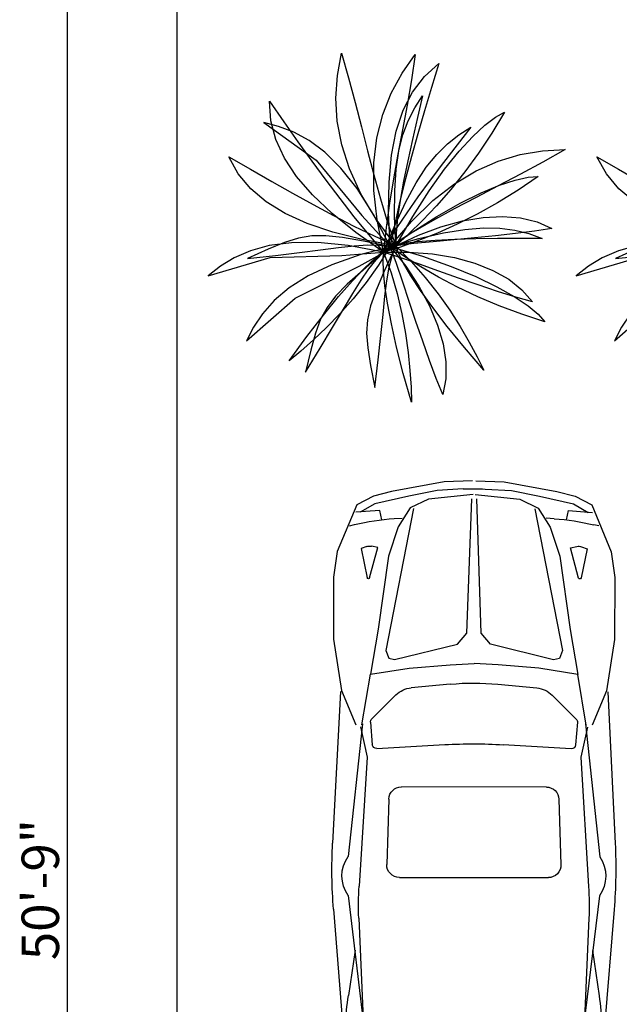
# Model space of a CAD drawing. Units: inches. Extents: x 3394 to 4794, y 965 to 1718.
# Tile 6 of 15: x 3394 to 3522, y 1338 to 1548. Entities that reach past the tile are written whole.
import ezdxf

# ---------------------------------------------------------------- set-up
doc = ezdxf.new("R2010")
doc.units = ezdxf.units.IN
for name, color, linetype, lineweight in [('A-ANNO-DIMS', 2, 'Continuous', 13), ('C-PRKG-VEHI', 8, 'Continuous', 13), ('C-PROP', 7, 'Continuous', 25), ('CAY', 94, 'Continuous', 13)]:
    doc.layers.add(name, color=color, linetype=linetype, lineweight=lineweight)
doc.layers.add('DIENHOA', color=3, linetype='Continuous')
doc.layers.add('L9012X$0', color=2, linetype='Continuous')
doc.styles.get("Standard").update_dxf_attribs({"font": 'arial.ttf'})
doc.dimstyles.new('ISO-25', dxfattribs={"dimtxt": 8, "dimasz": 2.5, "dimexe": 1.25, "dimexo": 0.625, "dimtad": 1, "dimlunit": 3, "dimtxsty": 'Standard', "dimcen": 2.5, "dimadec": 0, "dimazin": 0, "dimtfac": 1, "dimtmove": 0, "dimatfit": 3, "dimfxl": 1, "dimarcsym": 0})

# ---------------------------------------------------------------- blocks, each defined once
blk = doc.blocks.new('A1099DC')
at = {"color": 0, "linetype": 'ByBlock'}
for p, q in [((1279.298465, 804.448389), (2201.430588, 851.890505)), ((2602.736326, 846.078152), (3356.693814, 785.353187)), ((272.228253, 749.073842), (265.114727, 718.465169)), ((1475.52921, 670.226262), (2282.402739, 758.004075)), ((2519.280414, 756.817792), (3387.476361, 653.818028)), ((2851.341839, 715.213377), (3126.60716, 755.701993)), ((3488.458929, 772.663345), (3732.658862, 759.86454)), ((139.051458, 595.027331), (190.951238, 683.213377)), ((179.200345, 564.515703), (190.951238, 709.631982)), ((398.733388, 644.315148), (411.280494, 678.748261)), ((411.280494, 678.748261), (588.616917, 641.417897)), ((1482.852352, 674.283145), (1175.286956, 622.180789)), ((1494.603245, 682.841284), (1678.210958, 641.166865)), ((1678.210958, 641.166865), (2462.684993, 690.847736)), ((2656.476214, 692.831247), (3376.704709, 662.004075)), ((3376.704709, 662.004075), (3510.708679, 626.736433)), ((3909.27561, 688.812956), (3837.725727, 693.401722)), ((3867.794139, 700.329656), (3900.059395, 686.767505)), ((3921.162781, 527.618662), (3921.162781, 676.138994)), ((3925.383812, 676.122818), (3955.306409, 663.545364)), ((405.405047, 577.538958), (396.874865, 615.894428)), ((589.014326, 626.599587), (405.405047, 577.538958)), ((1300.814287, 466.658131), (1445.712032, 613.104998)), ((1465.665584, 620.56924), (1602.893878, 610.287296)), ((92.537504, 388.14361), (139.051458, 595.027331)), ((236.043912, 551.980927), (179.200345, 564.515703)), ((1626.354615, 583.507504), (1602.652901, 169.222264)), ((1933.148906, 509.557888), (2330.980062, 522.200075)), ((3522.252709, 492.345257), (3666.066199, 475.644444)), ((3704.596898, 536.993674), (3795.675135, 473.385795)), ((3841.786866, 503.451367), (3910.58243, 515.096797)), ((3901.001848, 514.780764), (3957.150905, 375.772812)), ((229.117398, 477.634662), (225.714299, 427.957563)), ((1860.238743, -448.635916), (1859.369151, 433.397797)), ((2409.60024, 445.938054), (2410.49349, -460.09121)), ((3493.960271, 465.734554), (3507.923021, 209.166865)), ((3839.396146, 426.841284), (3888.358202, 417.538958)), ((57.774444, 216.608726), (92.537504, 388.14361)), ((1235.045743, 136.116317), (1257.419842, 373.755108)), ((3753.293176, 397.789551), (3815.226005, 132.124765)), ((3857.610793, 379.525702), (3912.067615, 118.157673)), ((3888.358202, 417.538958), (3983.199613, 359.957848)), ((3983.199613, 359.957848), (4035.448301, 43.94997)), ((49.168662, 58.00681), (57.774444, 216.608726)), ((3507.923021, 209.166865), (3507.64153, -4.333678)), ((4019.086894, 150.376168), (4084.69605, 122.469191)), ((4084.69605, 122.469191), (4109.177079, 60.329656)), ((4109.177079, 60.329656), (4113.094043, -5.158716)), ((3508.347273, -221.154823), (3507.644805, -7.65525)), ((3983.920268, -371.008369), (4035.545755, -54.898082)), ((4109.306686, -71.132359), (4113.094514, -5.636391)), ((49.301278, -76.507426), (58.219773, -235.092064)), ((4084.948231, -133.320044), (4109.306686, -71.132359)), ((1235.330373, -152.586046), (1258.173002, -390.180259)), ((3754.088875, -409.293325), (3815.497749, -143.506937)), ((3858.370276, -390.823819), (3912.311631, -129.348921)), ((4019.394229, -161.356334), (4084.948231, -133.320044)), ((58.219773, -235.092064), (93.320996, -406.558069)), ((1627.520644, -599.204785), (1603.002095, -184.967086)), ((3494.890446, -477.749545), (3508.347273, -221.154823)), ((93.320996, -406.558069), (140.24279, -613.349673)), ((3889.19258, -428.776374), (3983.920268, -371.008369)), ((3902.027941, -525.993061), (3957.902795, -386.874665)), ((230.077082, -495.779641), (226.576036, -446.109349)), ((3840.248961, -438.175225), (3889.19258, -428.776374)), ((1301.750547, -482.997536), (1446.936772, -629.158411)), ((1934.168526, -524.650381), (2332.023837, -536.508105)), ((3523.2353, -504.304409), (3667.01558, -487.320059)), ((3705.667171, -548.593196), (3796.61981, -484.805853)), ((3842.790735, -514.780444), (3911.609128, -526.290202)), ((237.150178, -570.112104), (180.331436, -582.758939)), ((180.331436, -582.758939), (192.368445, -727.851766)), ((406.561378, -595.336142), (398.106841, -633.708356)), ((590.267037, -644.034637), (406.561378, -595.336142)), ((3922.214148, -538.79118), (3922.506998, -687.311224)), ((140.24279, -613.349673), (192.316354, -701.433212)), ((1484.19765, -690.263206), (1176.530118, -638.767405)), ((1466.905004, -636.583294), (1604.112757, -626.030785)), ((1495.965396, -698.798158), (1679.490579, -656.761786)), ((1679.490579, -656.761786), (2464.061049, -704.895745)), ((3378.022114, -674.249887), (3511.956283, -638.718087)), ((400.0214, -662.125356), (412.636377, -696.533662)), ((412.636377, -696.533662), (589.898847, -658.853701)), ((1476.866524, -686.22077), (2283.911563, -772.40743)), ((2520.786439, -770.754078), (3388.777604, -666.042617)), ((2657.855804, -706.497136), (3378.022114, -674.249887)), ((3910.644841, -700.0086), (3839.104145, -704.738438)), ((3869.186159, -711.60707), (3901.424611, -697.981326)), ((3926.727989, -687.286725), (3956.625729, -674.650294)), ((273.723073, -767.133288), (266.549207, -736.538701)), ((2852.765183, -728.494989), (3128.109803, -768.440762)), ((3489.994314, -784.688586), (3734.168535, -771.408296)), ((1280.900818, -820.829563), (2203.124693, -866.453338)), ((2604.418191, -859.849707), (3358.254477, -797.638217))]:
    blk.add_line(p, q, dxfattribs=at)
for points in [[(-0.000783, 0.794772), (5.385043, 172.701749), (63.649891, 493.818028), (92.537504, 603.957563), (144.437284, 705.166865), (428.417214, 824.236633), (585.095796, 846.190121), (961.406447, 846.190121), (1274.27399, 797.818028), (1482.852352, 709.631982)], [(83.345007, -3.206171), (111.32237, 268.957533), (164.563706, 379.583828), (279.999271, 453.709838), (456.549665, 511.628518), (901.254996, 574.918954), (1175.286956, 622.180789), (1137.52997, 385.548359), (1118.345181, 137.317882), (1109.829198, -8.358455)], [(168.178729, 359.003083), (1030.214866, 528.397865), (1077.798844, 510.531569), (1086.170082, 475.285426), (992.832238, 91.960378), (924.218938, 35.478085), (108.447994, 6.034416)], [(0.019119, -19.392451), (5.743899, -191.288474), (64.641806, -512.289243), (93.746535, -622.371603), (145.845778, -723.478374), (430.059935, -841.987962), (586.7815, -863.632471), (963.091723, -863.198028), (1275.863278, -814.209121), (1484.26735, -725.611974)], [(83.356858, -15.227176), (111.870816, -287.335185), (165.330179, -397.856284), (280.911681, -471.754535), (457.575935, -529.324983), (902.4055, -592.045995), (1176.530118, -638.767405), (1138.306616, -402.209884), (1118.632407, -154.017717), (1109.829198, -8.358455)], [(168.904615, -377.268451), (1031.273389, -545.270714), (1078.822046, -527.310627), (1087.123771, -492.048047), (993.030273, -108.907787), (924.305735, -52.560894), (108.478017, -24.418246)]]:
    blk.add_lwpolyline(points, dxfattribs=at)
for centre, radius, start, end in [((2358.037832, -2192.08357), 3048, 85.395244, 92.945173), ((2399.99649, 588.663508), 206.166238, 54.649181, 124.776949), ((1749.553982, 373.478072), 1524, 166.916578, 176.08111), ((3392.740754, -1053.630025), 1828.8, 86.999806, 98.367602), ((3718.678317, 475.802507), 284.405862, 57.329946, 87.182375), ((2578.271641, -1134.295865), 1828.8, 87.549126, 93.623712), ((4191.049821, 605.937201), 363.988953, 166.096081, 196.353514), ((3908.462781, 676.138994), 12.7, 0, 86.330429), ((3896.252417, 523.051998), 152.4, 46.38363, 67.20138), ((446.46332, 626.922805), 50.8, 159.97873, 192.538409), ((587.047263, 633.961317), 7.62, 284.960009, 78.112462), ((1463.767788, 595.240237), 25.4, 85.715073, 135.304647), ((1600.996082, 584.958293), 25.4, 356.725615, 85.715073), ((3355.555414, 37.211519), 609.6, 55.070043, 75.255062), ((3320.85101, 50.338397), 847.430844, 356.245089, 44.519453), ((3700.933354, 318.064082), 435.542335, 30.457681, 46.38363), ((3204.184594, 25.950693), 1011.814461, 358.069446, 30.457681), ((1935.569151, 433.396333), 76.2, 91.82012, 179.9989), ((2333.400307, 446.03852), 76.2, 359.924458, 91.82012), ((3519.322741, 467.114813), 25.4, 83.37601, 183.115039), ((3908.462781, 527.618662), 12.7, 279.607718, 0), ((1409.148822, 359.469565), 152.4, 135.304647, 174.62136), ((3654.346327, 374.722669), 101.6, 13.122645, 83.37601), ((3708.414764, 348.440256), 152.4, 11.769371, 55.070043), ((2752.335538, -6.739118), 1524, 174.62136, 185.491615), ((4645.676894, -4.872483), 3048, 176.725615, 183.38736), ((3221.54491, -6.276527), 609.6, 346.99033, 13.122645), ((3315.283499, -6.18411), 609.6, 348.343604, 11.769371), ((1266.577845, -8.050136), 1219.2, 176.894161, 183.218814), ((3734.73098, -5.770579), 304.8, 350.724636, 9.388339), ((3320.962449, -62.69553), 847.430844, 315.593523, 3.867886), ((3204.248172, -38.537915), 1011.814461, 329.655294, 2.043529), ((1409.873518, -375.595566), 152.4, 185.491615, 224.808328), ((3655.096735, -386.42159), 101.6, 276.736965, 346.99033), ((3709.113243, -360.032616), 152.4, 305.042932, 348.343604), ((1936.438592, -448.484202), 76.2, 180.114076, 268.292856), ((2334.293902, -460.341926), 76.2, 268.292856, 0.188517), ((3520.255588, -479.079792), 25.4, 176.997936, 276.736965), ((1750.305335, -388.625277), 1524, 184.031865, 193.196397), ((4192.255091, -616.577407), 363.988953, 163.759461, 194.016894), ((3909.514173, -538.816222), 12.7, 0.112975, 80.505257), ((3355.640902, -49.500248), 609.6, 284.857913, 305.042932), ((3701.571953, -329.671253), 435.542335, 313.729345, 329.655294), ((447.716945, -644.638934), 50.8, 167.574566, 200.134245), ((588.314493, -651.400231), 7.62, 282.000513, 75.152966), ((1464.957267, -611.258083), 25.4, 224.808328, 274.397903), ((1602.165021, -600.705574), 25.4, 274.397903, 3.38736), ((3897.294828, -534.273643), 152.4, 292.911596, 313.729345), ((2576.048678, 1120.472221), 1828.8, 266.489263, 272.563849), ((3909.807023, -687.336265), 12.7, 273.782546, 0.112975), ((2401.171182, -602.835323), 206.166238, 235.336026, 305.463794), ((3390.675263, 1041.412497), 1828.8, 261.745373, 273.113169), ((3719.627907, -487.374382), 284.405862, 272.930601, 302.78303), ((2353.729565, 2177.823616), 3048, 267.167802, 274.717731)]:
    blk.add_arc(centre, radius, start, end, dxfattribs=at)
blk = doc.blocks.new('VI')
at = {"layer": 'L9012X$0'}
blk.add_blockref('A1099DC', (0, 0), dxfattribs=at)
blk = doc.blocks.new('Cay03_mb')
at = {"layer": 'DIENHOA'}
for p, q in [((118.6, 555.3), (166.2, 599.1)), ((166.2, 599.1), (142.2, 519.4)), ((79.5, 503.7), (118.6, 555.3)), ((48.6, 443.6), (79.5, 503.7)), ((142.2, 519.4), (119, 441.7)), ((25.5, 374.3), (48.6, 443.6)), ((119, 441.7), (96.7, 365.6)), ((-365.2, 390.3), (-414.4, 402.8)), ((-414.4, 402.8), (-240.2, 277.8)), ((-314.9, 371.3), (-365.2, 390.3)), ((-263.5, 343.5), (-314.9, 371.3)), ((9.9, 295.3), (25.5, 374.3)), ((96.7, 365.6), (75.6, 290.6)), ((-211.2, 304.6), (-263.5, 343.5)), ((-158, 252.3), (-211.2, 304.6)), ((1.6, 205.7), (9.9, 295.3)), ((363.4, 275.4), (436.8, 297.2)), ((436.8, 297.2), (511, 309.6)), ((511, 309.6), (585.9, 313.5)), ((585.9, 313.5), (511.8, 271.4)), ((-240.2, 277.8), (-88.4, 94.9)), ((75.6, 290.6), (55.7, 216.3)), ((290.6, 243.2), (363.4, 275.4)), ((511.8, 271.4), (437.6, 231.5)), ((-104.2, 184.4), (-158, 252.3)), ((218.5, 199.8), (290.6, 243.2)), ((437.6, 231.5), (363.7, 192.9)), ((0.2, 104.9), (1.6, 205.7)), ((55.7, 216.3), (37.3, 142.1)), ((147, 144.1), (218.5, 199.8)), ((-49.6, 98.5), (-104.2, 184.4)), ((363.7, 192.9), (290.2, 154.9)), ((37.3, 142.1), (20.5, 67.6)), ((75.9, 75.2), (147, 144.1)), ((290.2, 154.9), (217.4, 116.6)), ((5.4, -7.8), (-49.6, 98.5)), ((5.4, -7.8), (0.2, 104.9)), ((217.4, 116.6), (145.5, 77.3)), ((-88.4, 94.9), (5.4, -7.8)), ((5.4, -7.8), (75.9, 75.2)), ((20.5, 67.6), (5.4, -7.8)), ((145.5, 77.3), (74.7, 36.1)), ((74.7, 36.1), (5.4, -7.8)), ((100.3, 18.4), (182.2, 37.2)), ((182.2, 37.2), (253, 48.9)), ((253, 48.9), (314.6, 54.1)), ((314.6, 54.1), (369.2, 53.3)), ((369.2, 53.3), (418.6, 46.8)), ((418.6, 46.8), (464.9, 35.2)), ((464.9, 35.2), (510, 19)), ((-345, 5.4), (-399.6, -17.1)), ((-298.6, 20.1), (-345, 5.4)), ((-254.7, 27.4), (-298.6, 20.1)), ((-208, 27.8), (-254.7, 27.4)), ((-152.7, 21.7), (-208, 27.8)), ((-83.4, 9.7), (-152.7, 21.7)), ((5.4, -7.8), (-83.4, 9.7)), ((5.4, -7.8), (100.3, 18.4)), ((46.3, 0.9), (5.4, -7.8)), ((96.7, 7.5), (46.3, 0.9)), ((155, 12.2), (96.7, 7.5)), ((219.6, 15.4), (155, 12.2)), ((289, 17.4), (219.6, 15.4)), ((361.6, 18.5), (289, 17.4)), ((435.8, 18.9), (361.6, 18.5)), ((510, 19), (435.8, 18.9)), ((-399.6, -17.1), (-468, -47.9)), ((-375.6, -37.8), (-295.3, -27.9)), ((-295.3, -27.9), (-225.8, -18.9)), ((-225.8, -18.9), (-165.8, -11.3)), ((-165.8, -11.3), (-114, -5.7)), ((-114, -5.7), (-69, -2.9)), ((-69, -2.9), (-29.6, -3.4)), ((-45.1, -46.3), (-16.5, -22.4)), ((5.4, -7.8), (-33.2, -69.5)), ((-29.6, -3.4), (5.4, -7.8)), ((-16.5, -22.4), (5.4, -7.8)), ((5.4, -7.8), (56.8, -73.3)), ((25.9, -64.4), (5.4, -7.8)), ((5.4, -7.8), (112.8, -40.3)), ((53.5, -41.6), (5.4, -7.8)), ((-468, -47.9), (-375.6, -37.8)), ((-79.8, -79.6), (-45.1, -46.3)), ((47, -125.9), (25.9, -64.4)), ((107, -75.7), (53.5, -41.6)), ((112.8, -40.3), (207.5, -73.8)), ((-120.2, -122.1), (-79.8, -79.6)), ((-33.2, -69.5), (-74.6, -127.3)), ((56.8, -73.3), (100.4, -139.1)), ((165.5, -109.6), (107, -75.7)), ((207.5, -73.8), (289.5, -107.6)), ((-165.9, -174.1), (-120.2, -122.1)), ((-74.6, -127.3), (-117.8, -181.1)), ((68.7, -190.6), (47, -125.9)), ((228.7, -142.8), (165.5, -109.6)), ((289.5, -107.6), (359.3, -141.1)), ((100.4, -139.1), (135.9, -204.3)), ((296, -174.7), (228.7, -142.8)), ((359.3, -141.1), (416.9, -173.5)), ((-216.3, -235.6), (-165.9, -174.1)), ((-117.8, -181.1), (-162.1, -230.9)), ((90.8, -256.6), (68.7, -190.6)), ((367.1, -204.8), (296, -174.7)), ((416.9, -173.5), (462.6, -204.2)), ((135.9, -204.3), (162.8, -268.3)), ((441.6, -232.7), (367.1, -204.8)), ((462.6, -204.2), (496.5, -232.5)), ((-271, -306.6), (-216.3, -235.6)), ((-162.1, -230.9), (-206.3, -276.5)), ((113.1, -322.2), (90.8, -256.6)), ((518.9, -257.7), (441.6, -232.7)), ((496.5, -232.5), (518.9, -257.7)), ((-206.3, -276.5), (-249.6, -317.8)), ((162.8, -268.3), (181, -330.4)), ((-329.5, -387.1), (-271, -306.6)), ((-249.6, -317.8), (-291, -354.7)), ((135.4, -385.6), (113.1, -322.2)), ((-291, -354.7), (-329.5, -387.1)), ((181, -330.4), (190, -390)), ((157.6, -445), (135.4, -385.6)), ((190, -390), (189.6, -446.3)), ((179.5, -498.7), (157.6, -445)), ((189.6, -446.3), (179.5, -498.7))]:
    blk.add_line(p, q, dxfattribs=at)
for points in [[(23.7, -5.4), (-41, 82.2), (-91.8, 167.1), (-129.7, 249.5), (-155.6, 329.6), (-170.2, 407.8), (-174.7, 484.2), (-169.8, 559.3), (-156.5, 633.1)], [(-156.5, 633.1), (-132.5, 551.3), (-110.5, 470), (-89.8, 389.2), (-69.6, 309), (-49, 229.4), (-27.1, 150.4), (-3.2, 72.1), (23.7, -5.4)], [(-16.4, -26.7), (-38.3, 80), (-48.9, 178.3), (-48.7, 269), (-38.5, 352.6), (-19.1, 429.7), (9, 501), (44.9, 567.1), (87.9, 628.5)], [(87.9, 628.5), (75.5, 544.2), (61.3, 461.2), (46.1, 379.1), (30.8, 297.8), (16.1, 216.9), (2.9, 136), (-8.3, 54.9), (-16.4, -26.7)], [(23.7, -5.4), (19.8, 93), (20.3, 177), (25, 248.5), (34, 309.8), (47.3, 362.7), (64.9, 409.3), (86.8, 451.7), (112.9, 491.9)], [(112.9, 491.9), (96, 419.7), (79.5, 347.4), (63.9, 276.5), (50, 208.4), (38.4, 144.8), (29.7, 86.9), (24.6, 36.3), (23.7, -5.4)], [(-395.6, 473.7), (-347.5, 405.6), (-300.6, 339.5), (-254.3, 275.1), (-208.3, 212.3), (-161.9, 150.9), (-114.8, 90.7), (-66.5, 31.6), (-16.4, -26.7)], [(-16.4, -26.7), (-108.3, 38.6), (-186.9, 101.7), (-252.4, 163.5), (-305.1, 224.4), (-345.4, 285.2), (-373.7, 346.6), (-390.4, 409.2), (-395.6, 473.7)], [(384.3, 437.5), (342.2, 367.8), (298.1, 301.7), (252.6, 239.4), (206.1, 181.1), (159.4, 127.2), (113, 78), (67.6, 33.6), (23.7, -5.4)], [(23.7, -5.4), (79.9, 91.7), (134.1, 176.2), (185.8, 248.4), (234.3, 308.7), (279, 357.3), (319.3, 394.8), (354.6, 421.4), (384.3, 437.5)], [(273.2, 387.3), (227.6, 328.8), (182.3, 270.1), (138.4, 212.3), (97.2, 156.4), (60, 103.4), (27.8, 54.6), (1.9, 10.8), (-16.4, -26.7)], [(-16.4, -26.7), (21.4, 64.2), (57, 140.3), (91.4, 203.3), (125.2, 255.1), (159.5, 297.5), (195, 332.5), (232.7, 361.8), (273.2, 387.3)], [(-530.5, 289.7), (-458.3, 248.1), (-387.9, 207.8), (-318.9, 168.7), (-250.8, 131.1), (-182.9, 94.8), (-114.9, 59.9), (-46.2, 26.5), (23.7, -5.4)], [(23.7, -5.4), (-87.2, 15.2), (-185, 39.6), (-270.3, 68.2), (-343.7, 101.4), (-405.9, 139.7), (-457.3, 183.5), (-498.7, 233.4), (-530.5, 289.7)], [(496.7, 224), (429.4, 178.4), (361.6, 136.9), (294.1, 99.5), (227.5, 66.1), (162.4, 36.7), (99.7, 11.5), (39.8, -9.7), (-16.4, -26.7)], [(-16.4, -26.7), (75.4, 37.9), (160.1, 91.8), (237.3, 135.7), (306.6, 170), (367.6, 195.4), (419.9, 212.5), (463.1, 221.9), (496.7, 224)], [(23.7, -5.4), (99.3, 29.7), (173.2, 57.1), (244.8, 76.7), (313.3, 88.3), (377.9, 91.8), (437.9, 87), (492.7, 73.8), (541.4, 52)], [(541.4, 52), (484.1, 42.9), (421.2, 34.8), (354.4, 27.6), (285.4, 20.9), (216.1, 14.5), (148.2, 8.1), (83.5, 1.6), (23.7, -5.4)], [(-16.4, -26.7), (-134, -4.7), (-235.3, 5.3), (-322, 4.7), (-395.9, -5), (-458.7, -22.3), (-512.3, -45.7), (-558.2, -73.6), (-598.4, -104.7)], [(-598.4, -104.7), (-392.7, -44.4), (-155, -37.4), (-16.4, -26.7)], [(-471.9, -320.3), (-310.5, -179.3), (-97.7, -73.3), (23.7, -5.4)], [(23.7, -5.4), (-92.3, -34.8), (-188.4, -68.2), (-266.9, -105.1), (-329.9, -144.9), (-379.7, -187), (-418.5, -230.7), (-448.5, -275.3), (-471.9, -320.3)], [(-276.2, -424.4), (-227.3, -345.4), (-185.7, -276.1), (-150, -215.7), (-119.1, -163.8), (-91.5, -119.5), (-66, -82.3), (-41.4, -51.6), (-16.4, -26.7)], [(-16.4, -26.7), (-84.9, -86), (-137, -133.1), (-175.8, -173), (-204.3, -210), (-225.5, -249.1), (-242.5, -294.7), (-258.4, -351.6), (-276.2, -424.4)], [(23.7, -5.4), (-13.6, -87.9), (-41.1, -152.6), (-59.6, -205), (-69.9, -250.7), (-72.8, -295), (-69.2, -343.6), (-59.7, -401.9), (-45.3, -475.5)], [(-45.3, -475.5), (-34.1, -383.2), (-25.4, -302.8), (-18.3, -233.1), (-12, -172.9), (-5.6, -121.2), (2, -76.8), (11.4, -38.5), (23.7, -5.4)], [(76.2, -524.2), (48.8, -428.5), (26.6, -341.7), (9.2, -264.1), (-3.6, -196.1), (-12.3, -138), (-17.1, -90.2), (-18.3, -53), (-16.4, -26.7)], [(-16.4, -26.7), (66.9, -26.6), (145.6, -32.7), (218.8, -44.9), (285.8, -63.1), (345.9, -87.1), (398.4, -116.6), (442.6, -151.6), (477.6, -191.8)], [(477.6, -191.8), (421.8, -176), (361.3, -156.9), (297.6, -135.5), (232.2, -112.6), (166.6, -89.4), (102.3, -66.6), (40.8, -45.4), (-16.4, -26.7)], [(-16.4, -26.7), (8.5, -95.1), (28.5, -163.3), (44.3, -230.6), (56.3, -296.1), (65, -359), (70.9, -418.5), (74.5, -473.9), (76.2, -524.2)], [(316.5, -418.1), (251.4, -342.8), (194.8, -273.3), (146.5, -210.2), (106.3, -153.8), (74.1, -104.7), (49.7, -63.4), (32.9, -30.1), (23.7, -5.4)], [(23.7, -5.4), (74.9, -57.1), (121.8, -110.6), (164.3, -165), (202.7, -219.4), (237, -272.9), (267.3, -324.5), (293.7, -373.2), (316.5, -418.1)]]:
    blk.add_lwpolyline(points, dxfattribs=at)
blk = doc.blocks.new('*D31')
at = {"layer": 'A-ANNO-DIMS', "color": 0, "lineweight": -2, "transparency": 16777216}
for p, q in [((3427.12, 1666.68), (3402.95, 1666.68)), ((3404.2, 1664.18), (3404.2, 1060.18)), ((3427.12, 1057.68), (3402.95, 1057.68))]:
    blk.add_line(p, q, dxfattribs=at)
at = {"layer": 'A-ANNO-DIMS', "color": 0, "transparency": 16777216}
for points in [[(3403.78, 1664.18), (3404.62, 1664.18), (3404.2, 1666.68)], [(3403.78, 1060.18), (3404.62, 1060.18), (3404.2, 1057.68)]]:
    blk.add_solid(points, dxfattribs=at)
at = {"layer": 'Defpoints', "color": 0, "transparency": 16777216}
for p in [(3427.74, 1666.68), (3404.2, 1057.68), (3427.74, 1057.68)]:
    blk.add_point(p, dxfattribs=at)
at = {"layer": 'A-ANNO-DIMS', "color": 0, "transparency": 16777216, "insert": (3399.49, 1362.18), "char_height": 8, "attachment_point": 5, "rotation": 90}
blk.add_mtext('50\'-9"', dxfattribs=at)

msp = doc.modelspace()

# ---------------------------------------------------------------- linework, layer by layer
at = {"layer": 'C-PROP'}
msp.add_line((3427.745, 1057.682), (3427.745, 1666.682), dxfattribs=at)

# ---------------------------------------------------------------- block references
at = {"layer": 'C-PRKG-VEHI', "xscale": -0.0351896714874634, "yscale": 0.0351896714874634, "zscale": 0.0351896714874634, "rotation": 90}
msp.add_blockref('VI', (3490.972, 1449.569), dxfattribs=at)
at = {"layer": 'CAY', "xscale": 0.0644925090660235, "yscale": 0.0644925090660235, "zscale": 0.0644925090660235}
for p in [(3472.978, 1500.195), (3551.739, 1500.195)]:
    msp.add_blockref('Cay03_mb', p, dxfattribs=at)

# ---------------------------------------------------------------- dimensions: what is measured, and where the dimension line sits
at = {"layer": 'A-ANNO-DIMS'}
dim = msp.add_linear_dim(base=(3404.201, 1057.682), p1=(3427.745, 1666.682), p2=(3427.745, 1057.682), angle=90, dimstyle='ISO-25', override={"dimclrd": 0, "dimclre": 0, "dimclrt": 0}, dxfattribs=at)
dim.commit()
dim.dimension.update_dxf_attribs({"geometry": '*D31', "text_midpoint": (3399.491, 1362.182)})

doc.saveas('drawing.dxf')
